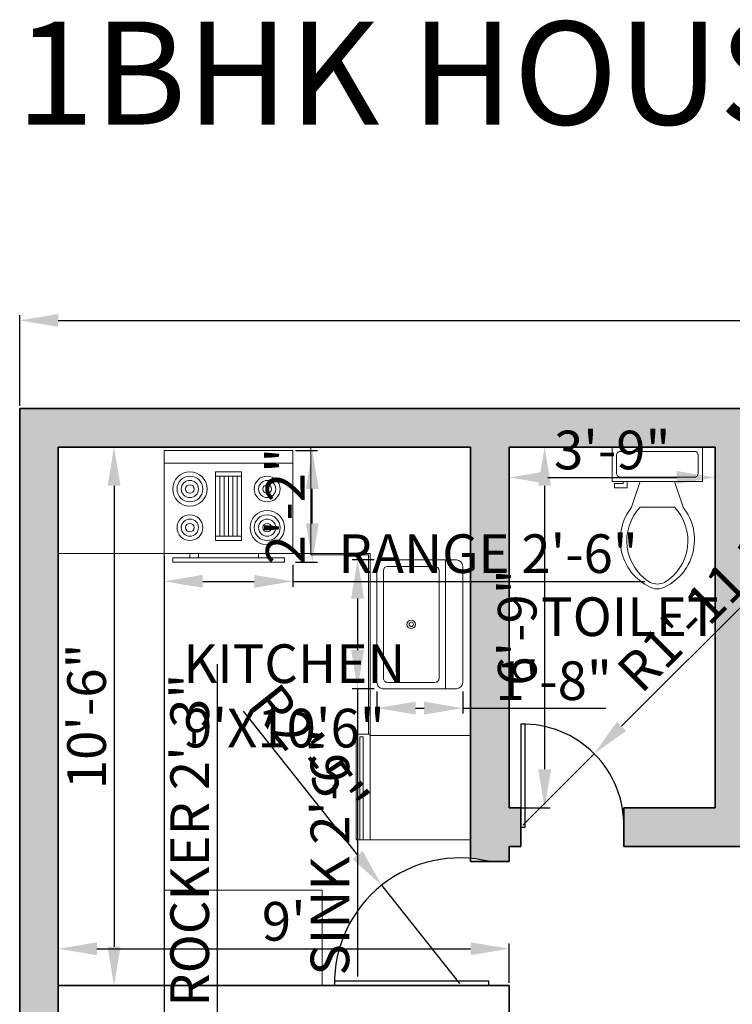
# Model space of a CAD drawing. Units: inches. Extents: x 39700 to 40173, y 40700 to 41139.
# Tile 2 of 4: x 39733 to 39899, y 40909 to 41139. Entities that reach past the tile are written whole.
import ezdxf

# ---------------------------------------------------------------- set-up
doc = ezdxf.new("R2010")
doc.units = ezdxf.units.IN
for name, color, linetype, lineweight in [('A-ANNO-DIMS', 2, 'Continuous', 18), ('A-ANNO-TEXT', 7, 'Continuous', 25), ('A-AREA-IDEN', 7, 'Continuous', 25), ('A-DOOR', 4, 'Continuous', 25), ('A-EQPM', 8, 'Continuous', 18), ('A-FLOR-CABN', 9, 'Continuous', 18), ('A-FLOR-FIXT', 9, 'Continuous', 18), ('A-WALL', 7, 'Continuous', 35)]:
    doc.layers.add(name, color=color, linetype=linetype, lineweight=lineweight)
doc.layers.add('A-WALL-PATT', color=251, linetype='Continuous', lineweight=13, true_color=0x636466)
doc.styles.get("Standard").update_dxf_attribs({"font": 'arial.ttf'})
doc.dimstyles.new('ISO-25', dxfattribs={"dimtxt": 9, "dimasz": 9, "dimexe": 1.25, "dimexo": 0.625, "dimtad": 1, "dimdec": 1, "dimrnd": 9, "dimlunit": 3, "dimtxsty": 'Standard', "dimcen": 2.5, "dimadec": 0, "dimazin": 0, "dimtfac": 1, "dimtdec": 1, "dimtmove": 0, "dimatfit": 3, "dimfxl": 1, "dimarcsym": 0})

# ---------------------------------------------------------------- blocks, each defined once
blk = doc.blocks.new('*D1')
at = {"layer": 'A-ANNO-DIMS', "color": 0, "lineweight": -2, "transparency": 16777216}
for p, q in [((39743.05, 41039.04), (39756.64, 41039.04)), ((39755.39, 41030.04), (39755.39, 40922.69)), ((39743.05, 40913.69), (39756.64, 40913.69))]:
    blk.add_line(p, q, dxfattribs=at)
at = {"layer": 'A-ANNO-DIMS', "color": 0, "transparency": 16777216}
for points in [[(39753.89, 41030.04), (39756.89, 41030.04), (39755.39, 41039.04)], [(39753.89, 40922.69), (39756.89, 40922.69), (39755.39, 40913.69)]]:
    blk.add_solid(points, dxfattribs=at)
at = {"layer": 'Defpoints', "color": 0, "transparency": 16777216}
for p in [(39742.42, 41039.04), (39742.42, 40913.69), (39755.39, 40913.69)]:
    blk.add_point(p, dxfattribs=at)
at = {"layer": 'A-ANNO-DIMS', "color": 0, "transparency": 16777216, "insert": (39750.17, 40976.37), "char_height": 9, "attachment_point": 5, "rotation": 90}
blk.add_mtext('10\'-6"', dxfattribs=at)
blk = doc.blocks.new('*D2')
at = {"layer": 'A-ANNO-DIMS', "color": 0, "lineweight": -2, "transparency": 16777216}
for p, q in [((39742.42, 40914.31), (39742.42, 40923.49)), ((39751.42, 40922.24), (39838.42, 40922.24)), ((39847.42, 40914.31), (39847.42, 40923.49))]:
    blk.add_line(p, q, dxfattribs=at)
at = {"layer": 'A-ANNO-DIMS', "color": 0, "transparency": 16777216}
for points in [[(39751.42, 40923.74), (39751.42, 40920.74), (39742.42, 40922.24)], [(39838.42, 40923.74), (39838.42, 40920.74), (39847.42, 40922.24)]]:
    blk.add_solid(points, dxfattribs=at)
at = {"layer": 'Defpoints', "color": 0, "transparency": 16777216}
for p in [(39847.42, 40922.24), (39742.42, 40913.69), (39847.42, 40913.69)]:
    blk.add_point(p, dxfattribs=at)
at = {"layer": 'A-ANNO-DIMS', "color": 0, "transparency": 16777216, "insert": (39794.92, 40927.46), "char_height": 9, "attachment_point": 5}
blk.add_mtext("9'", dxfattribs=at)
blk = doc.blocks.new('*D3')
at = {"layer": 'A-ANNO-DIMS', "color": 0, "lineweight": -2, "transparency": 16777216}
for p, q in [((39847.42, 41038.42), (39847.42, 41030.73)), ((39895.42, 41038.42), (39895.42, 41030.73)), ((39856.42, 41031.98), (39886.42, 41031.98))]:
    blk.add_line(p, q, dxfattribs=at)
at = {"layer": 'A-ANNO-DIMS', "color": 0, "transparency": 16777216}
for points in [[(39856.42, 41033.48), (39856.42, 41030.48), (39847.42, 41031.98)], [(39886.42, 41033.48), (39886.42, 41030.48), (39895.42, 41031.98)]]:
    blk.add_solid(points, dxfattribs=at)
at = {"layer": 'Defpoints', "color": 0, "transparency": 16777216}
for p in [(39847.42, 41039.04), (39895.42, 41039.04), (39895.42, 41031.98)]:
    blk.add_point(p, dxfattribs=at)
at = {"layer": 'A-ANNO-DIMS', "color": 0, "transparency": 16777216, "insert": (39871.42, 41037.2), "char_height": 9, "attachment_point": 5}
blk.add_mtext('3\'-9"', dxfattribs=at)
blk = doc.blocks.new('*D4')
at = {"layer": 'A-ANNO-DIMS', "color": 0, "lineweight": -2, "transparency": 16777216}
for p, q in [((39848.05, 41039.04), (39856.92, 41039.04)), ((39855.67, 41030.04), (39855.67, 40964.04)), ((39848.05, 40955.04), (39856.92, 40955.04))]:
    blk.add_line(p, q, dxfattribs=at)
at = {"layer": 'A-ANNO-DIMS', "color": 0, "transparency": 16777216}
for points in [[(39854.17, 41030.04), (39857.17, 41030.04), (39855.67, 41039.04)], [(39854.17, 40964.04), (39857.17, 40964.04), (39855.67, 40955.04)]]:
    blk.add_solid(points, dxfattribs=at)
at = {"layer": 'Defpoints', "color": 0, "transparency": 16777216}
for p in [(39847.42, 41039.04), (39847.42, 40955.04), (39855.67, 40955.04)]:
    blk.add_point(p, dxfattribs=at)
at = {"layer": 'A-ANNO-DIMS', "color": 0, "transparency": 16777216, "insert": (39850.45, 40997.04), "char_height": 9, "attachment_point": 5, "rotation": 90}
blk.add_mtext('6\'-9"', dxfattribs=at)
blk = doc.blocks.new('*D9')
at = {"layer": 'A-ANNO-DIMS', "color": 0, "lineweight": -2, "transparency": 16777216}
for p, q in [((39733.42, 41048.67), (39733.42, 41069.8)), ((40093.42, 41048.67), (40093.42, 41069.8)), ((39742.42, 41068.55), (40084.42, 41068.55))]:
    blk.add_line(p, q, dxfattribs=at)
at = {"layer": 'A-ANNO-DIMS', "color": 0, "transparency": 16777216}
for points in [[(39742.42, 41070.05), (39742.42, 41067.05), (39733.42, 41068.55)], [(40084.42, 41070.05), (40084.42, 41067.05), (40093.42, 41068.55)]]:
    blk.add_solid(points, dxfattribs=at)
at = {"layer": 'Defpoints', "color": 0, "transparency": 16777216}
for p in [(40093.42, 41068.55), (39733.42, 41048.04), (40093.42, 41048.04)]:
    blk.add_point(p, dxfattribs=at)
at = {"layer": 'A-ANNO-DIMS', "color": 0, "transparency": 16777216, "insert": (39913.42, 41073.77), "char_height": 9, "attachment_point": 5}
blk.add_mtext("30'", dxfattribs=at)
blk = doc.blocks.new('Range-Oven - 30 in top')
for p, q in [((0, -3), (30, -3)), ((12, -6), (18, -6)), ((13, -20), (13, -6)), ((14, -6), (14, -20)), ((15, -20), (15, -6)), ((16, -6), (16, -20)), ((17, -20), (17, -6)), ((18, -20), (12, -20)), ((6, -24), (6, -25)), ((8, -25), (8, -24)), ((22, -25), (22, -24)), ((24, -24), (24, -25))]:
    blk.add_line(p, q)
for points in [[(0, -24), (0, 0), (30, 0), (30, -24)], [(12, -21), (12, -5), (18, -5), (18, -21)], [(2, -26), (2, -25), (28, -25), (28, -26)]]:
    blk.add_lwpolyline(points, close=True)
for centre, radius in [((6, -9), 4), ((6, -9), 3), ((24, -9), 3), ((6, -9), 2), ((6, -9), 1), ((24, -9), 2), ((24, -9), 1), ((6, -18), 3), ((6, -18), 2), ((24, -18), 4), ((24, -18), 3), ((24, -18), 2), ((6, -18), 1), ((24, -18), 1)]:
    blk.add_circle(centre, radius)
blk = doc.blocks.new('Sink-single - 30 in top')
blk.add_line((-15, -3.999996), (15, -3.999996))
for points in [[(-13.5, 0), (13.5, 0)], [(-15, -18.499996), (-15, -1.5)], [(15, -1.5), (15, -18.499996)], [(-13.5, -17.499996), (-13.5, -6.499996)], [(-12.5, -5.499996), (12.5, -5.499996)], [(13.5, -6.499996), (13.5, -17.499996)], [(13.5, -19.999996), (-13.5, -19.999996)], [(12.5, -18.499996), (-12.5, -18.499996)]]:
    blk.add_lwpolyline(points)
for radius in [1, 0.5]:
    blk.add_circle((0, -11.999996), radius)
for centre, radius, start, end in [((-13.5, -1.5), 1.5, 90, 180), ((13.5, -1.5), 1.5, 0, 90), ((-12.5, -6.499996), 1, 90, 180), ((12.5, -6.499996), 1, 0, 90), ((-12.5, -17.499996), 1, 180, 270), ((12.5, -17.499996), 1, 270, 0), ((-13.5, -18.499996), 1.5, 180, 270), ((13.5, -18.499996), 1.5, 270, 0)]:
    blk.add_arc(centre, radius, start, end)
blk = doc.blocks.new('Toilet - top')
for p, q in [((9.5, -6), (9.5, -2)), ((-10, -8.5), (-8, -8.5)), ((-10, -9.5), (-10, -8.5)), ((-8, -8.5), (-8, -8)), ((-7, -8), (-7, -9.5)), ((-4, -8), (-6, -14)), ((4, -8), (6, -14)), ((-7, -9.5), (-10, -9.5)), ((4, -14), (-4, -14))]:
    blk.add_line(p, q)
blk.add_lwpolyline([(10.5, -8), (10.5, 0), (-10.5, 0), (-10.5, -8)], close=True)
for points in [[(-9.5, -2), (-9.5, -6)], [(8.5, -1), (-8.5, -1)], [(-8.5, -7), (8.5, -7)]]:
    blk.add_lwpolyline(points)
for centre, radius, start, end in [((-8.62, -1.88), 0.884, 81.8699, 188.1301), ((8.62, -1.88), 0.884, 351.8699, 98.1301), ((-8.62, -6.12), 0.884, 171.8699, 278.1301), ((8.62, -6.12), 0.884, 261.8699, 8.1301), ((3.52, -21.58), 12.17, 141.4691, 247.9714), ((4.2, -21.82), 11.33, 136.3677, 238.9468), ((-3.52, -21.58), 12.17, 292.0284, 38.5307), ((-4.2, -21.82), 11.33, 301.053, 43.6321), ((0, -27.88), 4, 245.7318, 294.2682), ((0, -29), 4, 254.8605, 285.1395)]:
    blk.add_arc(centre, radius, start, end)
blk = doc.blocks.new('*D26')
at = {"layer": 'A-ANNO-DIMS', "color": 0, "lineweight": -2, "transparency": 16777216}
for p, q in [((39767.06, 41011.67), (39767.06, 41006.54)), ((39797.06, 41011.67), (39797.06, 41006.54)), ((39776.06, 41007.79), (39788.06, 41007.79)), ((39797.06, 41007.79), (39878.98, 41007.79))]:
    blk.add_line(p, q, dxfattribs=at)
at = {"layer": 'A-ANNO-DIMS', "color": 0, "transparency": 16777216}
for points in [[(39776.06, 41009.29), (39776.06, 41006.29), (39767.06, 41007.79)], [(39788.06, 41009.29), (39788.06, 41006.29), (39797.06, 41007.79)]]:
    blk.add_solid(points, dxfattribs=at)
at = {"layer": 'Defpoints', "color": 0, "transparency": 16777216}
for p in [(39767.06, 41012.29), (39797.06, 41012.29), (39797.06, 41007.79)]:
    blk.add_point(p, dxfattribs=at)
at = {"layer": 'A-ANNO-DIMS', "color": 0, "transparency": 16777216, "insert": (39842.52, 41013.07), "char_height": 9, "attachment_point": 5}
blk.add_mtext('RANGE 2\'-6"', dxfattribs=at)
blk = doc.blocks.new('*D27')
at = {"layer": 'A-ANNO-DIMS', "color": 0, "lineweight": -2, "transparency": 16777216}
for p, q in [((39797.69, 41038.29), (39802.81, 41038.29)), ((39801.56, 41021.29), (39801.56, 41029.29)), ((39797.69, 41012.29), (39802.81, 41012.29))]:
    blk.add_line(p, q, dxfattribs=at)
at = {"layer": 'A-ANNO-DIMS', "color": 0, "transparency": 16777216}
for points in [[(39800.06, 41029.29), (39803.06, 41029.29), (39801.56, 41038.29)], [(39800.06, 41021.29), (39803.06, 41021.29), (39801.56, 41012.29)]]:
    blk.add_solid(points, dxfattribs=at)
at = {"layer": 'Defpoints', "color": 0, "transparency": 16777216}
for p in [(39797.06, 41038.29), (39801.56, 41038.29), (39797.06, 41012.29)]:
    blk.add_point(p, dxfattribs=at)
at = {"layer": 'A-ANNO-DIMS', "color": 0, "transparency": 16777216, "insert": (39796.42, 41025.29), "char_height": 9, "attachment_point": 5, "rotation": 90}
blk.add_mtext('2\'-2"', dxfattribs=at)
blk = doc.blocks.new('*D28')
at = {"layer": 'A-ANNO-DIMS', "color": 0, "lineweight": -2, "transparency": 16777216}
for p, q in [((39815.99, 41012.77), (39810.86, 41012.77)), ((39812.11, 41003.77), (39812.11, 40991.77)), ((39815.99, 40982.77), (39810.86, 40982.77)), ((39812.11, 40982.77), (39812.11, 40915.8))]:
    blk.add_line(p, q, dxfattribs=at)
at = {"layer": 'A-ANNO-DIMS', "color": 0, "transparency": 16777216}
for points in [[(39810.61, 41003.77), (39813.61, 41003.77), (39812.11, 41012.77)], [(39810.61, 40991.77), (39813.61, 40991.77), (39812.11, 40982.77)]]:
    blk.add_solid(points, dxfattribs=at)
at = {"layer": 'Defpoints', "color": 0, "transparency": 16777216}
for p in [(39816.61, 41012.77), (39812.11, 40982.77), (39816.61, 40982.77)]:
    blk.add_point(p, dxfattribs=at)
at = {"layer": 'A-ANNO-DIMS', "color": 0, "transparency": 16777216, "insert": (39806.83, 40944.79), "char_height": 9, "attachment_point": 5, "rotation": 90}
blk.add_mtext('SINK 2\'-6"', dxfattribs=at)
blk = doc.blocks.new('*D29')
at = {"layer": 'A-ANNO-DIMS', "color": 0, "lineweight": -2, "transparency": 16777216}
for p, q in [((39816.61, 40982.15), (39816.61, 40977.02)), ((39836.61, 40982.15), (39836.61, 40977.02)), ((39825.61, 40978.27), (39827.61, 40978.27)), ((39836.61, 40978.27), (39869.94, 40978.27))]:
    blk.add_line(p, q, dxfattribs=at)
at = {"layer": 'A-ANNO-DIMS', "color": 0, "transparency": 16777216}
for points in [[(39825.61, 40979.77), (39825.61, 40976.77), (39816.61, 40978.27)], [(39827.61, 40979.77), (39827.61, 40976.77), (39836.61, 40978.27)]]:
    blk.add_solid(points, dxfattribs=at)
at = {"layer": 'Defpoints', "color": 0, "transparency": 16777216}
for p in [(39816.61, 40982.77), (39836.61, 40982.77), (39836.61, 40978.27)]:
    blk.add_point(p, dxfattribs=at)
at = {"layer": 'A-ANNO-DIMS', "color": 0, "transparency": 16777216, "insert": (39857.78, 40983.49), "char_height": 9, "attachment_point": 5}
blk.add_mtext('1\'-8"', dxfattribs=at)
blk = doc.blocks.new('*D31')
at = {"layer": 'A-ANNO-DIMS', "color": 0, "lineweight": -2, "transparency": 16777216}
for p, q in [((39886.03, 40886.79), (39886.03, 40896.97)), ((39924.53, 40886.79), (39924.53, 40896.97)), ((39886.03, 40895.72), (39830.89, 40895.72)), ((39915.53, 40895.72), (39895.03, 40895.72))]:
    blk.add_line(p, q, dxfattribs=at)
at = {"layer": 'A-ANNO-DIMS', "color": 0, "transparency": 16777216}
for points in [[(39895.03, 40897.22), (39895.03, 40894.22), (39886.03, 40895.72)], [(39915.53, 40897.22), (39915.53, 40894.22), (39924.53, 40895.72)]]:
    blk.add_solid(points, dxfattribs=at)
at = {"layer": 'Defpoints', "color": 0, "transparency": 16777216}
for p in [(39886.03, 40895.72), (39886.03, 40886.16), (39924.53, 40886.16)]:
    blk.add_point(p, dxfattribs=at)
at = {"layer": 'A-ANNO-DIMS', "color": 0, "transparency": 16777216, "insert": (39853.96, 40901), "char_height": 9, "attachment_point": 5}
blk.add_mtext('3\'-2 1/2"', dxfattribs=at)
blk = doc.blocks.new('*D36')
at = {"layer": 'A-ANNO-DIMS', "color": 0, "lineweight": -2, "transparency": 16777216}
for p, q in [((39779.47, 40897.52), (39779.47, 40988.51)), ((39776.04, 40897.52), (39780.72, 40897.52)), ((39779.47, 40879.52), (39779.47, 40888.52)), ((39776.04, 40870.52), (39780.72, 40870.52))]:
    blk.add_line(p, q, dxfattribs=at)
at = {"layer": 'A-ANNO-DIMS', "color": 0, "transparency": 16777216}
for points in [[(39777.97, 40888.52), (39780.97, 40888.52), (39779.47, 40897.52)], [(39777.97, 40879.52), (39780.97, 40879.52), (39779.47, 40870.52)]]:
    blk.add_solid(points, dxfattribs=at)
at = {"layer": 'Defpoints', "color": 0, "transparency": 16777216}
for p in [(39775.42, 40897.52), (39779.47, 40897.52), (39775.42, 40870.52)]:
    blk.add_point(p, dxfattribs=at)
at = {"layer": 'A-ANNO-DIMS', "color": 0, "transparency": 16777216, "insert": (39774.18, 40947.51), "char_height": 9, "attachment_point": 5, "rotation": 90}
blk.add_mtext('ROCKER 2\'-3"', dxfattribs=at)
blk = doc.blocks.new('*D49')
at = {"layer": 'A-ANNO-DIMS', "color": 0, "lineweight": -2, "transparency": 16777216}
for p, q in [((39742.42, 41013.67), (39742.42, 40724.94)), ((39767.06, 41013.67), (39767.06, 40724.94)), ((39751.42, 40726.19), (39758.06, 40726.19)), ((39767.06, 40726.19), (39822.36, 40726.19))]:
    blk.add_line(p, q, dxfattribs=at)
at = {"layer": 'A-ANNO-DIMS', "color": 0, "transparency": 16777216}
for points in [[(39751.42, 40727.69), (39751.42, 40724.69), (39742.42, 40726.19)], [(39758.06, 40727.69), (39758.06, 40724.69), (39767.06, 40726.19)]]:
    blk.add_solid(points, dxfattribs=at)
at = {"layer": 'Defpoints', "color": 0, "transparency": 16777216}
for p in [(39742.42, 41014.29), (39767.06, 41014.29), (39767.06, 40726.19)]:
    blk.add_point(p, dxfattribs=at)
at = {"layer": 'A-ANNO-DIMS', "color": 0, "transparency": 16777216, "insert": (39799.21, 40731.47), "char_height": 9, "attachment_point": 5}
blk.add_mtext('2\'-0 1/2"', dxfattribs=at)
blk = doc.blocks.new('*D53')
at = {"layer": 'A-ANNO-DIMS', "color": 0, "lineweight": -2, "transparency": 16777216}
for p, q in [((39785.45, 40977.53), (39812.11, 40944.07)), ((39835.91, 40914.19), (39817.72, 40937.03))]:
    blk.add_line(p, q, dxfattribs=at)
at = {"layer": 'A-ANNO-DIMS', "color": 0, "transparency": 16777216}
blk.add_solid([(39813.28, 40945), (39810.94, 40943.13), (39817.72, 40937.03)], dxfattribs=at)
at = {"layer": 'Defpoints', "color": 0, "transparency": 16777216}
for p in [(39817.72, 40937.03), (39835.91, 40914.19)]:
    blk.add_point(p, dxfattribs=at)
at = {"layer": 'A-ANNO-DIMS', "color": 0, "transparency": 16777216, "insert": (39800.06, 40967.57), "char_height": 9, "attachment_point": 5, "rotation": 308.5424}
blk.add_mtext('R2\'-5"', dxfattribs=at)
blk = doc.blocks.new('*D54')
at = {"layer": 'A-ANNO-DIMS', "color": 0, "lineweight": -2, "transparency": 16777216}
for p, q in [((39923.61, 41024.06), (39873.58, 40974.03)), ((39850.6, 40951.04), (39867.22, 40967.66))]:
    blk.add_line(p, q, dxfattribs=at)
at = {"layer": 'A-ANNO-DIMS', "color": 0, "transparency": 16777216}
blk.add_solid([(39872.52, 40975.09), (39874.64, 40972.97), (39867.22, 40967.66)], dxfattribs=at)
at = {"layer": 'Defpoints', "color": 0, "transparency": 16777216}
for p in [(39867.22, 40967.66), (39850.6, 40951.04)]:
    blk.add_point(p, dxfattribs=at)
at = {"layer": 'A-ANNO-DIMS', "color": 0, "transparency": 16777216, "insert": (39898.05, 41005.96), "char_height": 9, "attachment_point": 5, "rotation": 44.999}
blk.add_mtext('R1\'-11 1/2"', dxfattribs=at)

msp = doc.modelspace()

# ---------------------------------------------------------------- hatches: boundary and pattern name
at = {"layer": 'A-WALL-PATT'}
h = msp.add_hatch(color=256, dxfattribs=at)
h.dxf.hatch_style = 1
h.paths.add_polyline_path([(39742.42, 41039.04), (39838.42, 41039.04), (39838.42, 40943.28, -0.039113), (39842.92, 40942.53), (39847.42, 40942.53), (39847.42, 40946.04), (39850.1, 40946.04), (39850.1, 40955.04), (39847.42, 40955.04), (39847.42, 41039.04), (39895.42, 41039.04), (39895.42, 40955.04), (39874.1, 40955.04), (39874.1, 40951.54, -0.010637), (39874.1, 40950.54), (39874.1, 40946.04), (39895.42, 40946.04), (39904.42, 40946.04), (39904.42, 41039.04), (40084.42, 41039.04), (40084.42, 40895.04), (39960.51, 40895.04), (39960.51, 40886.04), (40084.42, 40886.04), (40084.42, 40817.04), (40093.42, 40817.04), (40093.42, 41048.04), (39733.42, 41048.04), (39733.42, 40889.95), (39742.42, 40889.95)])
h.paths.add_polyline_path([(39742.42, 40841.95), (39733.42, 40841.95), (39733.42, 40817.06), (39737.92, 40817.06, -0.015901), (39740.88, 40817.06), (39742.42, 40817.06)], flags=17)
h.paths.add_polyline_path([(40093.42, 40757.04), (39796.66, 40757.04), (39796.66, 40748.04), (40093.42, 40748.04)])
h.paths.add_polyline_path([(39753.27, 40757.04), (39742.42, 40757.04), (39742.42, 40769.06), (39733.42, 40769.06), (39733.42, 40748.04), (39753.27, 40748.04)])
h.paths.add_polyline_path([(40084.42, 40826.04), (39960.51, 40826.04), (39960.51, 40817.04), (40084.42, 40817.04)], flags=17)
h.paths.add_polyline_path([(39969.51, 40859.86), (39960.51, 40859.86), (39960.51, 40852.78), (39969.51, 40852.78)], flags=17)
h.paths.add_polyline_path([(39969.51, 40886.04), (39960.51, 40886.04), (39960.51, 40881.75), (39969.51, 40881.75)], flags=17)
h.paths.add_polyline_path([(39852.31, 40989.98), (39900.82, 40989.98), (39900.82, 41008.52), (39852.31, 41008.52)], flags=25)

# ---------------------------------------------------------------- linework, layer by layer
at = {"layer": 'A-DOOR'}
for p, q in [((39851.1, 40974.54), (39850.1, 40974.54)), ((39850.1, 40974.54), (39850.1, 40955.04)), ((39851.1, 40950.54), (39851.1, 40974.54)), ((39850.1, 40950.54), (39851.1, 40950.54)), ((39842.71, 40914.69), (39806.71, 40914.69)), ((39806.71, 40914.69), (39806.71, 40913.69)), ((39842.71, 40913.69), (39842.71, 40914.69))]:
    msp.add_line(p, q, dxfattribs=at)
for centre, radius, start, end in [((39850.6, 40951.04), 23.51, 358.7811, 91.2189), ((39835.91, 40914.19), 29.2, 76.1042, 180.9811)]:
    msp.add_arc(centre, radius, start, end, dxfattribs=at)
at = {"layer": 'A-EQPM'}
for p, q in [((39814.88, 40972.24), (39811.81, 40972.24)), ((39811.81, 40972.24), (39811.81, 40947.61)), ((39815.07, 40947.61), (39815.07, 40971.93)), ((39811.81, 40947.61), (39815.07, 40947.61)), ((39838.42, 40947.61), (39815.07, 40947.61))]:
    msp.add_line(p, q, dxfattribs=at)
msp.add_lwpolyline([(39812.61, 40971.57), (39813.44, 40971.57), (39813.44, 40947.61), (39812.61, 40947.61)], close=True, dxfattribs=at)
at = {"layer": 'A-FLOR-CABN'}
for p, q in [((39801.19, 41039.04), (39801.19, 41014.29)), ((39742.42, 41014.29), (39815.07, 41014.29)), ((39767.06, 41014.29), (39767.06, 40935.87)), ((39801.19, 41014.29), (39801.19, 41014)), ((39801.19, 41014), (39814.69, 41014)), ((39814.69, 41014), (39814.69, 40972.24)), ((39815.07, 41014.29), (39815.07, 40971.93)), ((39814.69, 40972.24), (39815.07, 40972.24)), ((39815.07, 40971.93), (39838.42, 40971.93)), ((39767.06, 40935.87), (39803.85, 40935.87)), ((39803.85, 40935.87), (39803.85, 40913.69))]:
    msp.add_line(p, q, dxfattribs=at)
at = {"layer": 'A-WALL'}
for p, q in [((40093.42, 41048.04), (39733.42, 41048.04)), ((39733.42, 41048.04), (39733.42, 40817.06)), ((39742.42, 41039.04), (39742.42, 40817.06)), ((39838.42, 41039.04), (39742.42, 41039.04)), ((39838.42, 41039.04), (39838.42, 40942.53)), ((39847.42, 41039.04), (39847.42, 40955.04)), ((39895.42, 41039.04), (39847.42, 41039.04)), ((39895.42, 41039.04), (39895.42, 40955.04)), ((39850.1, 40955.04), (39847.42, 40955.04)), ((39850.1, 40955.04), (39850.1, 40946.04)), ((39895.42, 40955.04), (39874.1, 40955.04)), ((39874.1, 40955.04), (39874.1, 40946.04)), ((39850.1, 40946.04), (39847.42, 40946.04)), ((39847.42, 40946.04), (39847.42, 40942.53)), ((39895.42, 40946.04), (39874.1, 40946.04)), ((39904.42, 40946.04), (39895.42, 40946.04)), ((39847.42, 40942.53), (39838.42, 40942.53)), ((39742.42, 40913.69), (39847.42, 40913.69)), ((39847.42, 40913.69), (39847.42, 40904.69))]:
    msp.add_line(p, q, dxfattribs=at)

# ---------------------------------------------------------------- block references
at = {"layer": 'A-EQPM'}
msp.add_blockref('Range-Oven - 30 in top', (39767.06, 41038.29), dxfattribs=at)
at = {"layer": 'A-FLOR-FIXT'}
msp.add_blockref('Toilet - top', (39881.92, 41039.04), dxfattribs=at)
at = {"layer": 'A-FLOR-FIXT', "rotation": 270}
msp.add_blockref('Sink-single - 30 in top', (39836.61, 40997.77), dxfattribs=at)

# ---------------------------------------------------------------- texts
at = {"layer": 'A-ANNO-TEXT', "insert": (39732.57, 41138.14), "char_height": 24, "attachment_point": 1}
msp.add_mtext_dynamic_manual_height_columns('1BHK HOUSE FLOOR PLAN', width=457.4103, gutter_width=12.5, heights=[0], dxfattribs=at)
at = {"layer": 'A-AREA-IDEN', "char_height": 9, "attachment_point": 1}
for s, insert in [('TOILET', (39854.85, 41004.05)), ('KITCHEN\\P9\'X10\'6"', (39771.5, 40993.12))]:
    msp.add_mtext_dynamic_manual_height_columns(s, width=34.373, gutter_width=12.5, heights=[0], dxfattribs=dict(at, insert=insert))

# ---------------------------------------------------------------- dimensions: what is measured, and where the dimension line sits
at = {"layer": 'A-ANNO-DIMS'}
for base, p1, p2, override, picture, middle in [((40093.42, 41068.55), (39733.42, 41048.04), (40093.42, 41048.04), {"dimclrd": 0, "dimclre": 0, "dimclrt": 0}, '*D9', (39913.42, 41073.77)), ((39895.42, 41031.98), (39847.42, 41039.04), (39895.42, 41039.04), {"dimclrd": 0, "dimclre": 0, "dimclrt": 0}, '*D3', (39871.42, 41037.2)), ((39767.06, 40726.19), (39742.42, 41014.29), (39767.06, 41014.29), {"dimdec": 1, "dimlfac": 1, "dimrnd": 0, "dimzin": 1, "dimdsep": 46, "dimlunit": 4, "dimfrac": 2}, '*D49', (39799.21, 40731.47)), ((39836.61, 40978.27), (39816.61, 40982.77), (39836.61, 40982.77), {"dimdec": 1, "dimlfac": 1, "dimrnd": 0, "dimzin": 1, "dimdsep": 46, "dimlunit": 4, "dimfrac": 2}, '*D29', (39857.78, 40983.49)), ((39847.42, 40922.24), (39742.42, 40913.69), (39847.42, 40913.69), {"dimclrd": 0, "dimclre": 0, "dimclrt": 0}, '*D2', (39794.92, 40927.46))]:
    dim = msp.add_linear_dim(base=base, p1=p1, p2=p2, dimstyle='ISO-25', override=override, dxfattribs=at)
    dim.commit()
    dim.dimension.update_dxf_attribs({"geometry": picture, "text_midpoint": middle})
for base, p1, p2, angle, override, picture, middle in [((39755.3939, 40913.6878), (39742.4234, 41039.0443), (39742.4234, 40913.6878), 90, {"dimclrd": 0, "dimclre": 0, "dimclrt": 0}, '*D1', (39750.1738, 40976.366)), ((39855.67, 40955.04), (39847.42, 41039.04), (39847.42, 40955.04), 90, {"dimclrd": 0, "dimclre": 0, "dimclrt": 0}, '*D4', (39850.45, 40997.04)), ((39801.56, 41038.29), (39797.06, 41012.29), (39797.06, 41038.29), 90, {"dimdec": 1, "dimlfac": 1, "dimrnd": 0, "dimzin": 1, "dimdsep": 46, "dimlunit": 4, "dimfrac": 2}, '*D27', (39796.42, 41025.29)), ((39886.03, 40895.72), (39924.53, 40886.16), (39886.03, 40886.16), 180, {"dimdec": 1, "dimlfac": 1, "dimrnd": 0, "dimzin": 1, "dimdsep": 46, "dimlunit": 4, "dimfrac": 2}, '*D31', (39853.96, 40901))]:
    dim = msp.add_linear_dim(base=base, p1=p1, p2=p2, angle=angle, dimstyle='ISO-25', override=override, dxfattribs=at)
    dim.commit()
    dim.dimension.update_dxf_attribs({"geometry": picture, "text_midpoint": middle})
for center, mpoint, picture, middle in [((39850.6, 40951.04), (39867.22, 40967.66), '*D54', (39898.05, 41005.96)), ((39835.91, 40914.19), (39817.72, 40937.03), '*D53', (39800.06, 40967.57))]:
    dim = msp.add_radius_dim(center=center, mpoint=mpoint, dimstyle='ISO-25', override={"dimdec": 1, "dimlfac": 1, "dimrnd": 0, "dimzin": 1, "dimdsep": 46, "dimlunit": 4, "dimfrac": 2}, dxfattribs=at)
    dim.commit()
    dim.dimension.update_dxf_attribs({"geometry": picture, "text_midpoint": middle})
dim = msp.add_linear_dim(base=(39797.06, 41007.79), p1=(39767.06, 41012.29), p2=(39797.06, 41012.29), text='RANGE <>', dimstyle='ISO-25', override={"dimdec": 1, "dimlfac": 1, "dimrnd": 0, "dimzin": 1, "dimdsep": 46, "dimlunit": 4, "dimfrac": 2}, dxfattribs=at)
dim.commit()
dim.dimension.update_dxf_attribs({"geometry": '*D26', "text_midpoint": (39842.52, 41013.07)})
for base, p1, p2, angle, text, picture, middle in [((39812.11, 40982.77), (39816.61, 41012.77), (39816.61, 40982.77), 270, 'SINK <>', '*D28', (39806.83, 40944.79)), ((39779.47, 40897.52), (39775.42, 40870.52), (39775.42, 40897.52), 90, 'ROCKER <>', '*D36', (39774.18, 40947.51))]:
    dim = msp.add_linear_dim(base=base, p1=p1, p2=p2, angle=angle, text=text, dimstyle='ISO-25', override={"dimdec": 1, "dimlfac": 1, "dimrnd": 0, "dimzin": 1, "dimdsep": 46, "dimlunit": 4, "dimfrac": 2}, dxfattribs=at)
    dim.commit()
    dim.dimension.update_dxf_attribs({"geometry": picture, "text_midpoint": middle})

doc.saveas('drawing.dxf')
